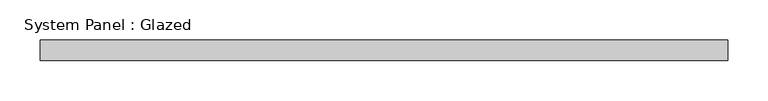
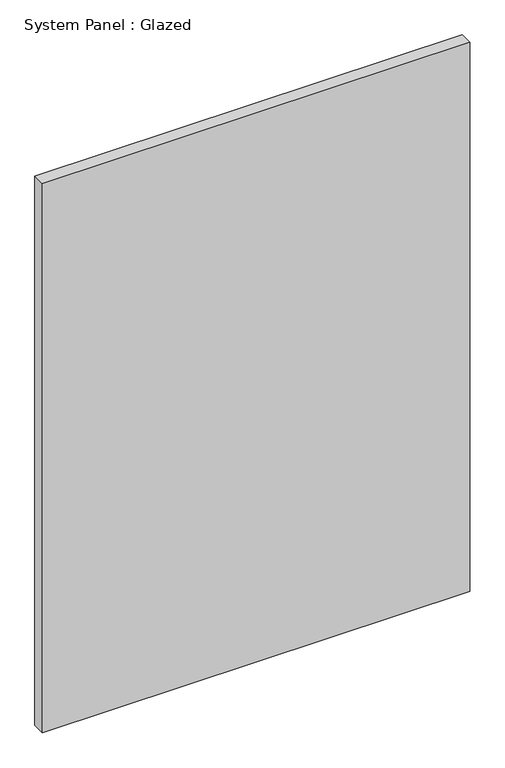
"""IFC4 building model written with IfcOpenShell, lengths in millimetres: plate geometry, System Panel : Glazed."""

from ifc_helpers import new_model, si_unit, origin, origin_with_axes, place, context, project, spatial, polyline, outline, extrude, source, transform, mapped, element, save


def system_panel_glazed_11b37e3b(model_context):
    return source(origin(), model_context, "Body", "SweptSolid", [
        extrude(outline(polyline([(425.45, 19.05), (-425.45, 19.05), (-425.45, 44.45), (425.45, 44.45), (425.45, 19.05)])), origin_with_axes(), (0.0, 0.0, 1.0), 1155.7),
    ])


if __name__ == "__main__":
    model = new_model("IFC4")
    model_context = context("Model", 3, world=origin())
    ifc_project = project(units=[si_unit("LENGTHUNIT", "METRE", prefix="MILLI")], contexts=[model_context])
    site = spatial("IfcSite", under=ifc_project)
    building = spatial("IfcBuilding", under=site)
    placement = place(None, origin())
    system_panel_glazed_shape = system_panel_glazed_11b37e3b(model_context)
    element("IfcPlate", 1, ObjectType="System Panel : Glazed", at=placement, inside=building, context=model_context, shape_type="MappedRepresentation", body=[
        mapped(system_panel_glazed_shape, transform((0.0, 0.0, 0.0), x_axis=(1.0, 0.0, 0.0), y_axis=(0.0, 1.0, 0.0), z_axis=(0.0, 0.0, 1.0))),
    ])
    save(model, "model.ifc")

# Revit data of these elements
# Type "System Panel : Glazed"
#   Construction Type Id = "GSP4R"
#   Analytic Construction = "1/8 in Pilkington single glazing"
#   Visual Light Transmittance = 0.9
#   Solar Heat Gain Coefficient = 0.86
#   Heat Transfer Coefficient (U) = 1.18115 BTU/(h·ft²·°F)
# Element 1 (IfcPlate, "System Panel : Glazed")
#   Materials on its faces: "Glass"
# Materials
#   "Glass": class "Glass", colour RGB 0 128 192, transparency 0.75, Description = "Soda Lime Glass", Cost = 0
